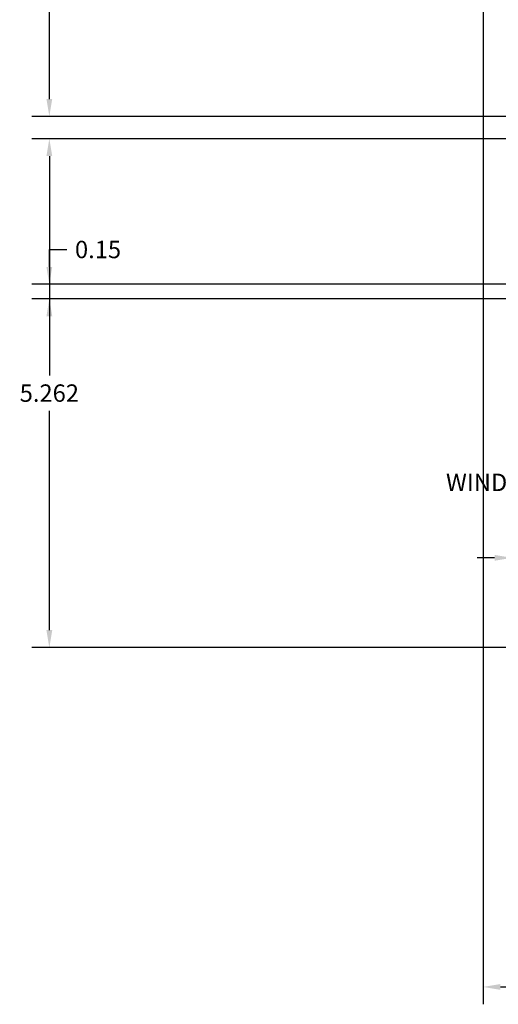
# Model space of a CAD drawing. Units: metres. Extents: x 2031 to 2061.8, y 1886.4 to 1909.8.
# Tile 1 of 10: x 2031.4 to 2036.4, y 1886.4 to 1896.6. Entities that reach past the tile are written whole.
import ezdxf

# ---------------------------------------------------------------- set-up
doc = ezdxf.new("R2010")
doc.units = ezdxf.units.M
doc.layers.add('A-ANNO-DIMS', color=2, linetype='Continuous', lineweight=18)
doc.styles.get("Standard").update_dxf_attribs({"font": 'arial.ttf'})
doc.dimstyles.get("Standard").update_dxf_attribs({"dimtxt": 0.18, "dimasz": 0.18, "dimexe": 0.18, "dimexo": 0.0625, "dimgap": 0.09, "dimtad": 0, "dimtih": 1, "dimtoh": 1, "dimdec": 4, "dimzin": 0, "dimdsep": 46, "dimtxsty": 'Standard', "dimcen": 0.09, "dimadec": 0, "dimazin": 0, "dimtfac": 1, "dimtdec": 4, "dimtofl": 0, "dimtmove": 0, "dimatfit": 3, "dimfxl": 1, "dimtolj": 1, "dimtzin": 0, "dimarcsym": 0})

# ---------------------------------------------------------------- blocks, each defined once
blk = doc.blocks.new('*D20')
at = {"layer": 'A-ANNO-DIMS', "color": 0, "lineweight": -2, "transparency": 16777216}
for p, q in [((2036.826, 1892.387), (2037.123, 1892.387)), ((2036.943, 1892.207), (2036.943, 1891.97)), ((2036.943, 1891.367), (2036.943, 1891.603)), ((2036.826, 1891.187), (2037.123, 1891.187))]:
    blk.add_line(p, q, dxfattribs=at)
at = {"layer": 'A-ANNO-DIMS', "color": 0, "transparency": 16777216}
for points in [[(2036.913, 1892.207), (2036.973, 1892.207), (2036.943, 1892.387)], [(2036.913, 1891.367), (2036.973, 1891.367), (2036.943, 1891.187)]]:
    blk.add_solid(points, dxfattribs=at)
at = {"layer": 'Defpoints', "color": 0, "transparency": 16777216}
for p in [(2036.763, 1892.387), (2036.943, 1892.387), (2036.763, 1891.187)]:
    blk.add_point(p, dxfattribs=at)
at = {"layer": 'A-ANNO-DIMS', "color": 0, "transparency": 16777216, "insert": (2036.943, 1891.787), "char_height": 0.18, "attachment_point": 5}
blk.add_mtext('\\A1;WINDOW W1 1 TYP.', dxfattribs=at)
blk = doc.blocks.new('*D21')
at = {"layer": 'A-ANNO-DIMS', "color": 0, "lineweight": -2, "transparency": 16777216}
for p, q in [((2036.533, 1891.124), (2036.533, 1890.827)), ((2036.763, 1891.124), (2036.763, 1890.827)), ((2036.353, 1891.007), (2036.173, 1891.007)), ((2036.943, 1891.007), (2037.123, 1891.007))]:
    blk.add_line(p, q, dxfattribs=at)
at = {"layer": 'A-ANNO-DIMS', "color": 0, "transparency": 16777216}
for points in [[(2036.353, 1891.037), (2036.353, 1890.977), (2036.533, 1891.007)], [(2036.943, 1891.037), (2036.943, 1890.977), (2036.763, 1891.007)]]:
    blk.add_solid(points, dxfattribs=at)
at = {"layer": 'Defpoints', "color": 0, "transparency": 16777216}
for p in [(2036.533, 1891.187), (2036.763, 1891.187), (2036.763, 1891.007)]:
    blk.add_point(p, dxfattribs=at)
at = {"layer": 'A-ANNO-DIMS', "color": 0, "transparency": 16777216, "insert": (2037.581, 1891.007), "char_height": 0.18, "attachment_point": 5}
blk.add_mtext('\\A1;0 TYP.', dxfattribs=at)
blk = doc.blocks.new('*D44')
at = {"layer": 'A-ANNO-DIMS', "color": 0, "lineweight": -2, "transparency": 16777216}
for p, q in [((2036.233, 1900.72), (2036.233, 1886.39)), ((2056.454, 1889.993), (2056.454, 1886.39)), ((2036.413, 1886.57), (2045.949, 1886.57)), ((2056.274, 1886.57), (2046.738, 1886.57))]:
    blk.add_line(p, q, dxfattribs=at)
at = {"layer": 'A-ANNO-DIMS', "color": 0, "transparency": 16777216}
for points in [[(2036.413, 1886.6), (2036.413, 1886.54), (2036.233, 1886.57)], [(2056.274, 1886.6), (2056.274, 1886.54), (2056.454, 1886.57)]]:
    blk.add_solid(points, dxfattribs=at)
at = {"layer": 'Defpoints', "color": 0, "transparency": 16777216}
for p in [(2036.233, 1900.782), (2056.454, 1890.056), (2056.454, 1886.57)]:
    blk.add_point(p, dxfattribs=at)
at = {"layer": 'A-ANNO-DIMS', "color": 0, "transparency": 16777216, "insert": (2046.343, 1886.57), "char_height": 0.18, "attachment_point": 5}
blk.add_mtext('\\A1;20.22', dxfattribs=at)
blk = doc.blocks.new('*D51')
at = {"layer": 'A-ANNO-DIMS', "color": 0, "lineweight": -2, "transparency": 16777216}
for p, q in [((2036.901, 1899.371), (2031.565, 1899.371)), ((2031.745, 1899.191), (2031.745, 1897.653)), ((2031.745, 1895.751), (2031.745, 1897.289)), ((2036.901, 1895.571), (2031.565, 1895.571))]:
    blk.add_line(p, q, dxfattribs=at)
at = {"layer": 'A-ANNO-DIMS', "color": 0, "transparency": 16777216}
for points in [[(2031.715, 1899.191), (2031.775, 1899.191), (2031.745, 1899.371)], [(2031.715, 1895.751), (2031.775, 1895.751), (2031.745, 1895.571)]]:
    blk.add_solid(points, dxfattribs=at)
at = {"layer": 'Defpoints', "color": 0, "transparency": 16777216}
for p in [(2031.745, 1899.371), (2036.963, 1899.371), (2036.963, 1895.571)]:
    blk.add_point(p, dxfattribs=at)
at = {"layer": 'A-ANNO-DIMS', "color": 0, "transparency": 16777216, "insert": (2031.745, 1897.471), "char_height": 0.18, "attachment_point": 5}
blk.add_mtext('\\A1;3.8', dxfattribs=at)
blk = doc.blocks.new('*D54')
at = {"layer": 'A-ANNO-DIMS', "color": 0, "lineweight": -2, "transparency": 16777216}
for p, q in [((2036.671, 1895.341), (2031.565, 1895.341)), ((2031.745, 1895.161), (2031.745, 1892.892)), ((2031.745, 1890.259), (2031.745, 1892.528)), ((2036.471, 1890.079), (2031.565, 1890.079))]:
    blk.add_line(p, q, dxfattribs=at)
at = {"layer": 'A-ANNO-DIMS', "color": 0, "transparency": 16777216}
for points in [[(2031.715, 1895.161), (2031.775, 1895.161), (2031.745, 1895.341)], [(2031.715, 1890.259), (2031.775, 1890.259), (2031.745, 1890.079)]]:
    blk.add_solid(points, dxfattribs=at)
at = {"layer": 'Defpoints', "color": 0, "transparency": 16777216}
for p in [(2036.733, 1895.341), (2031.745, 1890.079), (2036.533, 1890.079)]:
    blk.add_point(p, dxfattribs=at)
at = {"layer": 'A-ANNO-DIMS', "color": 0, "transparency": 16777216, "insert": (2031.745, 1892.71), "char_height": 0.18, "attachment_point": 5}
blk.add_mtext('\\A1;5.262', dxfattribs=at)
blk = doc.blocks.new('*D61')
at = {"layer": 'A-ANNO-DIMS', "color": 0, "lineweight": -2, "transparency": 16777216}
for p, q in [((2031.745, 1894.015), (2031.745, 1894.195)), ((2031.745, 1894.195), (2031.925, 1894.195)), ((2052.128, 1893.835), (2031.565, 1893.835)), ((2051.978, 1893.685), (2031.565, 1893.685)), ((2031.745, 1893.505), (2031.745, 1893.325))]:
    blk.add_line(p, q, dxfattribs=at)
at = {"layer": 'A-ANNO-DIMS', "color": 0, "transparency": 16777216}
for points in [[(2031.715, 1894.015), (2031.775, 1894.015), (2031.745, 1893.835)], [(2031.715, 1893.505), (2031.775, 1893.505), (2031.745, 1893.685)]]:
    blk.add_solid(points, dxfattribs=at)
at = {"layer": 'Defpoints', "color": 0, "transparency": 16777216}
for p in [(2031.745, 1893.835), (2052.19, 1893.835), (2052.04, 1893.685)]:
    blk.add_point(p, dxfattribs=at)
at = {"layer": 'A-ANNO-DIMS', "color": 0, "transparency": 16777216, "insert": (2032.249, 1894.195), "char_height": 0.18, "attachment_point": 5}
blk.add_mtext('\\A1;0.15', dxfattribs=at)

msp = doc.modelspace()

# ---------------------------------------------------------------- dimensions: what is measured, and where the dimension line sits
at = {"layer": 'A-ANNO-DIMS'}
dim = msp.add_linear_dim(base=(2056.4539, 1886.5702), p1=(2036.2328, 1900.7824), p2=(2056.4539, 1890.0556), dimstyle='Standard', override={"dimdec": 2, "dimlfac": 1, "dimrnd": 0, "dimzin": 0, "dimdsep": 46, "dimlunit": 2}, dxfattribs=at)
dim.commit()
dim.dimension.update_dxf_attribs({"geometry": '*D44', "text_midpoint": (2046.3433, 1886.5702)})
for base, p1, p2, override, picture, middle in [((2031.7448, 1899.3712), (2036.9632, 1895.5712), (2036.9632, 1899.3712), {"dimdec": 1, "dimlfac": 1, "dimrnd": 0, "dimzin": 0, "dimdsep": 46, "dimlunit": 2}, '*D51', (2031.7448, 1897.4712)), ((2031.7448, 1890.0791), (2036.7332, 1895.3412), (2036.5332, 1890.0791), {"dimdec": 3, "dimlfac": 1, "dimrnd": 0, "dimzin": 0, "dimdsep": 46, "dimlunit": 2}, '*D54', (2031.7448, 1892.7101)), ((2031.7448, 1893.8348), (2052.04, 1893.6848), (2052.19, 1893.8348), {"dimdec": 2, "dimlfac": 1, "dimrnd": 0, "dimzin": 0, "dimdsep": 46, "dimlunit": 2}, '*D61', (2032.2492, 1894.1948))]:
    dim = msp.add_linear_dim(base=base, p1=p1, p2=p2, angle=90, dimstyle='Standard', override=override, dxfattribs=at)
    dim.commit()
    dim.dimension.update_dxf_attribs({"geometry": picture, "text_midpoint": middle})
dim = msp.add_linear_dim(base=(2036.9432, 1892.3865), p1=(2036.7632, 1891.1865), p2=(2036.7632, 1892.3865), angle=90, text='WINDOW W1 <> TYP.', dimstyle='Standard', override={"dimdec": 0, "dimlfac": 1, "dimrnd": 0, "dimzin": 0, "dimdsep": 46, "dimlunit": 2}, dxfattribs=at)
dim.commit()
dim.dimension.update_dxf_attribs({"geometry": '*D20', "text_midpoint": (2036.9432, 1891.7865)})
dim = msp.add_linear_dim(base=(2036.7632, 1891.0065), p1=(2036.5332, 1891.1865), p2=(2036.7632, 1891.1865), text='<> TYP.', dimstyle='Standard', override={"dimdec": 0, "dimlfac": 1, "dimrnd": 0, "dimzin": 0, "dimdsep": 46, "dimlunit": 2}, dxfattribs=at)
dim.commit()
dim.dimension.update_dxf_attribs({"geometry": '*D21', "text_midpoint": (2037.5814, 1891.0065)})

doc.saveas('drawing.dxf')
